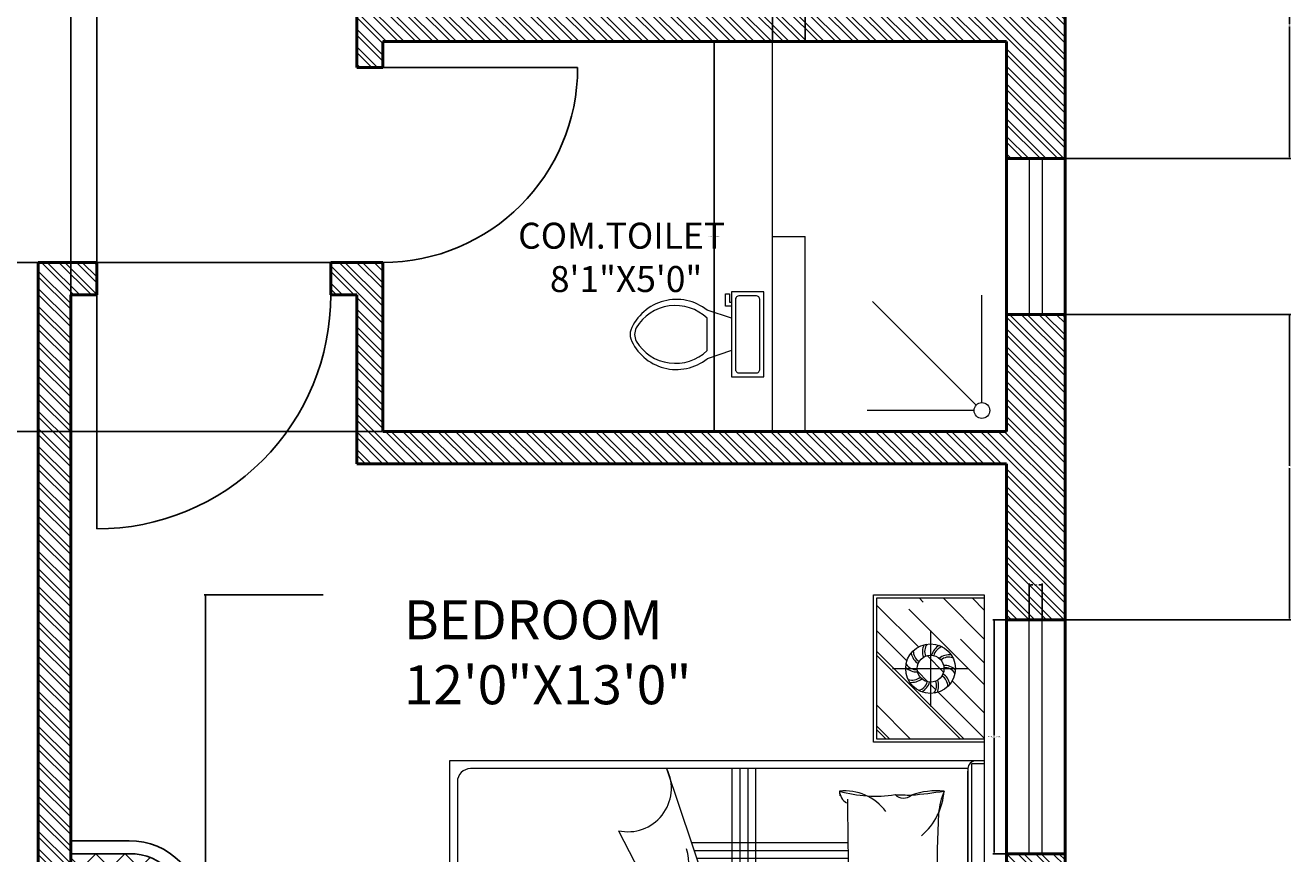
# Model space of a CAD drawing. Units: inches. Extents: x 10696 to 11614, y 5787 to 6498.
# Tile 3 of 9: x 10898 to 11093, y 5992 to 6120. Entities that reach past the tile are written whole.
import ezdxf

# ---------------------------------------------------------------- set-up
doc = ezdxf.new("R2010")
doc.units = ezdxf.units.IN
for name, color, linetype, lineweight in [('A-ANNO-DIMS', 2, 'Continuous', 18), ('A-AREA-IDEN', 7, 'Continuous', 25), ('A-DOOR', 3, 'Continuous', 25), ('A-FLOR-CASE', 32, 'Continuous', 25), ('A-FLOR-CASE-PATT', 252, 'Continuous', 13), ('A-FLOR-FIXT', 9, 'Continuous', 20), ('A-FURN', 8, 'Continuous', 18), ('A-GLAZ', 4, 'Continuous', 20), ('A-WALL', 7, 'Continuous', 50), ('A-WALL-PATT', 252, 'Continuous', 13)]:
    doc.layers.add(name, color=color, linetype=linetype, lineweight=lineweight)
doc.styles.get("Standard").update_dxf_attribs({"font": 'arial.ttf'})
doc.dimstyles.get("Standard").update_dxf_attribs({"dimtxt": 0.18, "dimasz": 0.18, "dimexe": 0.18, "dimexo": 0.0625, "dimgap": 0.09, "dimtad": 0, "dimtih": 1, "dimtoh": 1, "dimdec": 4, "dimzin": 0, "dimdsep": 46, "dimtxsty": 'Standard', "dimcen": 0.09, "dimadec": 0, "dimazin": 0, "dimtfac": 1, "dimtdec": 4, "dimtofl": 0, "dimtmove": 0, "dimatfit": 3, "dimfxl": 1, "dimtolj": 1, "dimtzin": 0, "dimarcsym": 0})

# ---------------------------------------------------------------- blocks, each defined once
blk = doc.blocks.new('A$C64B41DC1')
for p, q in [((0, 2.5079), (2.9903, 2.5079)), ((0, 2.0879), (0, 2.5079)), ((0.012, 2.4618), (0.0581, 2.5079)), ((0.012, 2.3515), (0.1684, 2.5079)), ((0.012, 2.0999), (0.012, 2.5079)), ((0.0543, 2.2213), (0.3409, 2.5079)), ((0.1689, 2.4179), (0.2589, 2.5079)), ((0.3265, 2.386), (0.4484, 2.5079)), ((0.3699, 2.3332), (0.5445, 2.5079)), ((0.548, 2.5079), (0.548, 2.0999)), ((0.56, 2.5079), (0.56, 2.0879)), ((0.6301, 2.5079), (0.6301, 0.4779)), ((0.6401, 2.461), (0.6401, 2.5079)), ((0.6401, 2.5079), (2.344, 2.5079)), ((2.344, 2.5079), (2.3601, 2.5079)), ((2.344, 2.5079), (2.344, 2.461)), ((2.3601, 2.5079), (2.3601, 2.4761)), ((2.3601, 0.4779), (2.3601, 2.5079)), ((2.4303, 2.5079), (2.4303, 2.0879)), ((2.4423, 2.5079), (2.4423, 2.0999)), ((2.4423, 2.3333), (2.6169, 2.5079)), ((2.4423, 2.2145), (2.7357, 2.5079)), ((2.705, 2.398), (2.8149, 2.5079)), ((2.7691, 2.3772), (2.8998, 2.5079)), ((2.7819, 2.3646), (2.9252, 2.5079)), ((2.9783, 2.0999), (2.9783, 2.5079)), ((2.9903, 2.0879), (2.9903, 2.5079)), ((2.344, 2.461), (0.6401, 2.461)), ((2.4423, 2.404), (2.5354, 2.4971)), ((0.2157, 2.0999), (0.548, 2.4322)), ((0.2299, 2.0999), (0.548, 2.418)), ((0.2804, 2.1597), (0.2804, 2.4481)), ((0.6601, 2.4461), (1.4951, 2.4461)), ((0.6601, 2.4461), (0.6601, 0.5579)), ((1.4951, 2.4461), (0.6697, 2.4461)), ((2.3301, 2.4461), (1.4951, 2.4461)), ((2.3301, 0.5579), (2.3301, 2.4461)), ((2.7099, 2.1597), (2.7099, 2.4481)), ((2.7914, 2.1846), (2.9783, 2.3715)), ((0.2311, 2.2906), (0.2937, 2.3532)), ((0.3405, 2.3039), (0.3605, 2.3238)), ((2.5849, 2.2779), (2.6158, 2.3088)), ((2.6158, 2.3088), (2.6313, 2.3243)), ((2.6674, 2.2756), (2.7382, 2.3464)), ((2.7249, 2.3076), (2.7512, 2.3339)), ((0.012, 2.261), (0.0275, 2.2765)), ((0.0404, 2.0999), (0.1982, 2.2578)), ((0.1362, 2.3039), (0.4246, 2.3039)), ((0.2905, 2.2539), (0.3304, 2.2938)), ((2.8541, 2.3039), (2.5657, 2.3039)), ((2.7746, 2.0999), (2.9783, 2.3036)), ((2.9144, 2.2312), (2.9783, 2.2951)), ((0.1365, 2.0999), (0.251, 2.2144)), ((0.4194, 2.0999), (0.548, 2.2285)), ((2.4423, 2.1353), (2.5382, 2.2312)), ((2.4918, 2.0999), (2.6366, 2.2447)), ((2.7831, 2.0999), (2.8678, 2.1846)), ((2.8962, 2.0999), (2.9783, 2.182)), ((0.4986, 2.0999), (0.548, 2.1493)), ((0.5127, 2.0999), (0.548, 2.1352)), ((0.56, 2.0879), (0, 2.0879)), ((0.548, 2.0999), (0.012, 2.0999)), ((2.4303, 2.0879), (2.9903, 2.0879)), ((2.4423, 2.0999), (2.9783, 2.0999)), ((2.5172, 2.0999), (2.5269, 2.1096)), ((0.9415, 1.9902), (0.9415, 1.3975)), ((0.9715, 1.9906), (0.9715, 1.4076)), ((1.0015, 1.991), (1.0015, 1.4177)), ((1.0315, 1.9916), (1.0315, 1.4279)), ((2.3349, 1.8678), (0.6613, 1.3029)), ((0.8956, 1.1191), (2.3349, 1.8678)), ((1.6636, 1.6412), (0.6601, 1.6412)), ((1.5748, 1.6112), (0.6601, 1.6112)), ((2.3665, 1.295), (2.3665, 1.3839)), ((2.377, 1.295), (2.3822, 1.3891)), ((2.4032, 1.295), (2.4032, 1.3839)), ((2.4346, 1.295), (2.4346, 1.3839)), ((2.4451, 1.295), (2.4503, 1.3891)), ((2.4774, 1.2957), (2.4774, 1.3837)), ((2.5, 1.295), (2.5, 1.3839)), ((2.5105, 1.295), (2.5157, 1.3891)), ((2.5367, 1.295), (2.5367, 1.3839)), ((2.5471, 1.295), (2.5524, 1.3891)), ((2.5681, 1.295), (2.5681, 1.3839)), ((2.5918, 1.295), (2.5918, 1.3839)), ((2.6346, 1.2957), (2.6346, 1.3837)), ((2.6362, 1.2957), (2.6467, 1.3839)), ((2.6729, 1.295), (2.6624, 1.3839)), ((2.6938, 1.295), (2.6938, 1.3839)), ((2.7043, 1.295), (2.7095, 1.3891)), ((2.7127, 1.2957), (2.7232, 1.3839)), ((2.7253, 1.295), (2.7253, 1.3839)), ((2.7494, 1.295), (2.7389, 1.3839)), ((2.7718, 1.295), (2.7718, 1.3839)), ((2.7959, 1.295), (2.7854, 1.3839)), ((2.8146, 1.2957), (2.8146, 1.3837)), ((2.8146, 1.2957), (2.8146, 1.3837)), ((2.8282, 1.295), (2.8282, 1.3839)), ((2.8282, 1.295), (2.8282, 1.3839)), ((2.8523, 1.295), (2.8418, 1.3839)), ((2.8523, 1.295), (2.8418, 1.3839)), ((2.8653, 1.2966), (2.8688, 1.3861)), ((2.8711, 1.2957), (2.8711, 1.3837)), ((2.8711, 1.2957), (2.8875, 1.3822)), ((2.8765, 1.2958), (2.9132, 1.3758)), ((2.8893, 1.3011), (2.9394, 1.3636)), ((2.8713, 1.2927), (2.954, 1.3315)), ((2.8717, 1.2884), (2.9588, 1.3058)), ((2.3601, 1.2873), (2.8639, 1.2873)), ((2.8639, 1.2873), (2.8639, 0.1018)), ((2.8716, 1.2565), (2.9605, 1.2669)), ((2.8723, 1.2489), (2.9603, 1.2489)), ((2.8744, 1.2817), (2.9603, 1.2869)), ((2.3601, 1.2233), (2.7999, 1.2233)), ((2.7999, 1.2233), (2.7999, 0.1658)), ((2.8716, 1.2212), (2.9605, 1.2212)), ((2.8716, 1.1947), (2.9605, 1.2052)), ((2.3601, 1.1913), (2.7679, 1.1912)), ((2.7679, 1.1912), (2.7679, 0.1978)), ((2.8716, 1.181), (2.9605, 1.1705)), ((2.8716, 1.1595), (2.9605, 1.1595)), ((2.8723, 1.1872), (2.9603, 1.1872)), ((2.8716, 1.133), (2.9605, 1.1435)), ((2.8716, 1.1193), (2.9605, 1.1088)), ((2.8723, 1.1255), (2.9603, 1.1255)), ((2.8716, 1.1035), (2.9605, 1.093)), ((2.8716, 1.0965), (2.9605, 1.0965)), ((2.8716, 1.086), (2.9657, 1.0913)), ((2.8716, 1.0756), (2.9605, 1.0756)), ((2.8716, 1.0491), (2.9605, 1.0596)), ((2.8723, 1.0858), (2.9605, 1.0753)), ((2.8716, 1.0354), (2.9605, 1.0249)), ((2.8723, 1.0416), (2.9603, 1.0416)), ((2.8723, 0.9987), (2.9605, 1.0092)), ((2.8723, 0.985), (2.9605, 0.9745)), ((2.8723, 0.9735), (2.9603, 0.9735)), ((2.8716, 0.9346), (2.9605, 0.9241)), ((2.8723, 0.9408), (2.9603, 0.9408)), ((2.8723, 0.8979), (2.9605, 0.9084)), ((2.8723, 0.8726), (2.9603, 0.8726)), ((2.8723, 0.8505), (2.9603, 0.8505)), ((2.8716, 0.7885), (2.9605, 0.799)), ((2.8716, 0.7818), (2.9657, 0.787)), ((2.8716, 0.7503), (2.9657, 0.7556)), ((2.8716, 0.7204), (2.9605, 0.7309)), ((2.8723, 0.7571), (2.9605, 0.7466)), ((2.8716, 0.6995), (2.9605, 0.6995)), ((2.8716, 0.689), (2.9657, 0.6838)), ((2.8716, 0.6576), (2.9657, 0.6523)), ((2.8716, 0.6471), (2.9605, 0.6471)), ((2.8716, 0.5903), (2.9605, 0.6007)), ((2.882, 0.5582), (2.9657, 0.5536)), ((0.7101, 0.5079), (2.2801, 0.5079)), ((2.8716, 0.4877), (2.9603, 0.4877)), ((2.8909, 0.5263), (2.9657, 0.5222)), ((2.8928, 0.5169), (2.9605, 0.5169)), ((0.6301, 0.4779), (2.3601, 0.4779)), ((1.2465, 0.4625), (1.1576, 0.452)), ((1.2465, 0.4365), (1.1577, 0.4365)), ((1.2542, 0.1018), (1.2542, 0.4779)), ((1.3182, 0.1658), (1.3182, 0.4779)), ((1.3502, 0.1978), (1.3502, 0.4779)), ((2.8716, 0.4625), (2.9605, 0.452)), ((2.8716, 0.4365), (2.9603, 0.4365)), ((1.2465, 0.3746), (1.1576, 0.3851)), ((2.8716, 0.3746), (2.9605, 0.3851)), ((1.2465, 0.3684), (1.1577, 0.3684)), ((2.8716, 0.3684), (2.9603, 0.3684)), ((1.2355, 0.3092), (1.1576, 0.3)), ((1.2285, 0.3357), (1.1577, 0.3357)), ((2.8826, 0.3092), (2.9605, 0.3)), ((2.8896, 0.3357), (2.9603, 0.3357)), ((1.2457, 0.2423), (1.1576, 0.2319)), ((1.2457, 0.2676), (1.1577, 0.2676)), ((2.8723, 0.2676), (2.9603, 0.2676)), ((2.8723, 0.2423), (2.9605, 0.2319)), ((1.2465, 0.2057), (1.1576, 0.2161)), ((2.7679, 0.1978), (1.3502, 0.1978)), ((2.8716, 0.2057), (2.9605, 0.2161)), ((1.2465, 0.1742), (1.1524, 0.169)), ((1.2465, 0.1847), (1.1576, 0.1847)), ((2.7999, 0.1658), (1.3182, 0.1658)), ((2.8716, 0.1847), (2.9605, 0.1847)), ((2.8716, 0.1742), (2.9657, 0.169)), ((1.2465, 0.1428), (1.1524, 0.1376)), ((1.2465, 0.1334), (1.1524, 0.1281)), ((1.2465, 0.1323), (1.1576, 0.1323)), ((1.2465, 0.1323), (1.1576, 0.1323)), ((1.2465, 0.1), (1.1576, 0.1105)), ((1.2465, 0.1229), (1.1588, 0.1168)), ((1.2464, 0.1007), (1.1592, 0.0833)), ((1.2468, 0.0964), (1.1641, 0.0576)), ((2.8639, 0.1018), (1.2542, 0.1018)), ((2.8713, 0.0964), (2.954, 0.0576)), ((2.8716, 0.1428), (2.9657, 0.1376)), ((2.8716, 0.1334), (2.9657, 0.1281)), ((2.8716, 0.1323), (2.9605, 0.1323)), ((2.8716, 0.1229), (2.9593, 0.1168)), ((2.8717, 0.1007), (2.9588, 0.0833)), ((2.8744, 0.1074), (2.9603, 0.1022)), ((1.2288, 0.088), (1.1787, 0.0255)), ((1.2415, 0.0933), (1.2049, 0.0133)), ((1.247, 0.0934), (1.2306, 0.0069)), ((1.2527, 0.0925), (1.2493, 0.003)), ((1.2658, 0.0941), (1.2762, 0.0052)), ((1.2899, 0.0941), (1.2899, 0.0052)), ((1.2999, 0.0941), (1.3051, 0)), ((1.3313, 0.0941), (1.3365, 0)), ((1.3523, 0.0941), (1.3575, 0)), ((1.3804, 0.0941), (1.3699, 0.0052)), ((1.4119, 0.0934), (1.4223, 0.0052)), ((1.4485, 0.0941), (1.438, 0.0052)), ((1.48, 0.0941), (1.4852, 0)), ((1.5114, 0.0941), (1.5166, 0)), ((1.5323, 0.0941), (1.5376, 0)), ((1.5638, 0.0941), (1.5638, 0.0105)), ((1.6021, 0.0941), (1.6021, 0.0052)), ((1.6336, 0.0941), (1.6336, 0.0052)), ((1.6702, 0.0941), (1.6702, 0.0052)), ((1.7017, 0.0941), (1.7017, 0.0052)), ((1.7122, 0.0941), (1.7174, 0)), ((1.7445, 0.0934), (1.7445, 0.0054)), ((1.7698, 0.0934), (1.7803, 0.0052)), ((1.8065, 0.0941), (1.796, 0.0052)), ((1.8274, 0.0941), (1.8274, 0.0052)), ((1.8379, 0.0941), (1.8431, 0)), ((1.8746, 0.0941), (1.8798, 0)), ((1.8955, 0.0941), (1.8955, 0.0052)), ((1.906, 0.0941), (1.9113, 0)), ((1.9384, 0.0934), (1.9384, 0.0054)), ((1.9609, 0.0941), (1.9609, 0.0052)), ((1.9636, 0.0934), (1.9741, 0.0052)), ((1.9714, 0.0941), (1.9766, 0)), ((1.9976, 0.0941), (1.9976, 0.0052)), ((2.0081, 0.0941), (2.0133, 0)), ((2.029, 0.0941), (2.029, 0.0052)), ((2.0395, 0.0941), (2.0447, 0)), ((2.0797, 0.0941), (2.0797, 0.0052)), ((2.0902, 0.0941), (2.0954, 0)), ((2.1216, 0.0941), (2.1269, 0)), ((2.1412, 0.0941), (2.1412, 0.0052)), ((2.1517, 0.0941), (2.1569, 0)), ((2.1831, 0.0941), (2.1884, 0)), ((2.2093, 0.0941), (2.2093, 0.0052)), ((2.2198, 0.0941), (2.225, 0)), ((2.2512, 0.0941), (2.2565, 0)), ((2.2603, 0.0934), (2.2707, 0.0052)), ((2.2969, 0.0941), (2.2864, 0.0052)), ((2.3089, 0.0934), (2.3193, 0.0052)), ((2.3455, 0.0941), (2.3351, 0.0052)), ((2.3665, 0.0941), (2.3665, 0.0052)), ((2.377, 0.0941), (2.3822, 0)), ((2.4032, 0.0941), (2.4032, 0.0052)), ((2.4346, 0.0941), (2.4346, 0.0052)), ((2.4451, 0.0941), (2.4503, 0)), ((2.4774, 0.0934), (2.4774, 0.0054)), ((2.5, 0.0941), (2.5, 0.0052)), ((2.5105, 0.0941), (2.5157, 0)), ((2.5367, 0.0941), (2.5367, 0.0052)), ((2.5471, 0.0941), (2.5524, 0)), ((2.5681, 0.0941), (2.5681, 0.0052)), ((2.5918, 0.0941), (2.5918, 0.0052)), ((2.6346, 0.0934), (2.6346, 0.0054)), ((2.6362, 0.0934), (2.6467, 0.0052)), ((2.6729, 0.0941), (2.6624, 0.0052)), ((2.6938, 0.0941), (2.6938, 0.0052)), ((2.7043, 0.0941), (2.7095, 0)), ((2.7127, 0.0934), (2.7232, 0.0052)), ((2.7253, 0.0941), (2.7253, 0.0052)), ((2.7494, 0.0941), (2.7389, 0.0052)), ((2.7718, 0.0941), (2.7718, 0.0052)), ((2.7959, 0.0941), (2.7854, 0.0052)), ((2.8146, 0.0934), (2.8146, 0.0054)), ((2.8282, 0.0941), (2.8282, 0.0052)), ((2.8523, 0.0941), (2.8418, 0.0052)), ((2.8653, 0.0925), (2.8688, 0.003)), ((2.8711, 0.0934), (2.8875, 0.0069)), ((2.8765, 0.0933), (2.9132, 0.0133)), ((2.8893, 0.088), (2.9394, 0.0255))]:
    blk.add_line(p, q)
at = {"ltscale": 10}
for p, q in [((1.4859, 1.5812), (0.6601, 1.5812)), ((1.397, 1.5512), (0.6601, 1.5512))]:
    blk.add_line(p, q, dxfattribs=at)
for centre, radius in [((0.2804, 2.3039), 0.0942), ((0.2804, 2.3039), 0.051), ((2.7099, 2.3039), 0.0942), ((2.7099, 2.3039), 0.051)]:
    blk.add_circle(centre, radius)
for centre, radius, start, end in [((0.6601, 2.4761), 0.03, 180, 270), ((2.3301, 2.4761), 0.03, 270, 0), ((0.2887, 2.3745), 0.0605, 172.17, 218.4897), ((0.2828, 2.3731), 0.0462, 160.3002, 220.538), ((0.3286, 2.3561), 0.0605, 136.17, 182.4897), ((0.3231, 2.3585), 0.0462, 124.3002, 184.538), ((0.3501, 2.3178), 0.0605, 100.17, 146.4897), ((0.347, 2.323), 0.0462, 88.3002, 148.538), ((1.0526, 2.3302), 0.3085, 175.3048, 198.6942), ((-0.8702, 2.0941), 1.6364, 4.8098, 9.1892), ((0.8579, 2.6278), 0.2948, 247.5179, 264.267), ((0.728, 2.111), 0.245, 40.4189, 85.9871), ((1.6986, 2.3355), 0.1943, 174.11, 233.4289), ((1.1481, 2.2311), 0.3783, 353.4947, 19.1867), ((1.6871, 3.192), 0.8561, 257.7438, 273.6284), ((1.4882, 2.111), 0.245, 40.4189, 85.9871), ((1.8674, 1.9709), 0.3878, 68.2026, 108.9817), ((2.6433, 2.323), 0.0462, 31.462, 91.6998), ((2.6402, 2.3178), 0.0605, 33.5103, 79.83), ((2.6672, 2.3585), 0.0462, 355.462, 55.6998), ((2.6617, 2.3561), 0.0605, 357.5103, 43.83), ((2.7075, 2.3731), 0.0462, 319.462, 19.6998), ((2.7016, 2.3745), 0.0605, 321.5103, 7.83), ((0.2457, 2.3659), 0.0605, 208.17, 254.4897), ((0.2417, 2.3614), 0.0462, 196.3002, 256.538), ((0.3449, 2.2742), 0.0605, 64.17, 110.4897), ((0.3455, 2.2802), 0.0462, 52.3002, 112.538), ((1.0164, 5.7096), 3.3803, 266.8134, 276.1602), ((1.3963, 2.1044), 0.245, 94.0129, 139.5811), ((1.1858, 2.3288), 0.1943, 306.5711, 5.89), ((1.5348, 2.2652), 0.1767, 151.7736, 201.6983), ((2.1269, 2.1044), 0.245, 94.0129, 139.5811), ((2.0342, 2.4856), 0.1563, 261.5958, 298.9092), ((1.9165, 2.3288), 0.1943, 333.7371, 5.89), ((2.6058, 2.2028), 0.517, 163.6046, 172.3273), ((2.6448, 2.2802), 0.0462, 67.462, 127.6998), ((2.6454, 2.2742), 0.0605, 69.5103, 115.83), ((2.7486, 2.3614), 0.0462, 283.462, 343.6998), ((2.7446, 2.3659), 0.0605, 285.5103, 331.83), ((0.2153, 2.3276), 0.0462, 232.3002, 292.538), ((0.2158, 2.3336), 0.0605, 244.17, 290.4897), ((0.2138, 2.2848), 0.0462, 268.3002, 328.538), ((0.2779, 2.2347), 0.0462, 340.3002, 40.538), ((0.272, 2.2333), 0.0605, 352.17, 38.4897), ((0.3191, 2.2464), 0.0462, 16.3002, 76.538), ((0.3151, 2.2419), 0.0605, 28.17, 74.4897), ((2.6752, 2.2419), 0.0605, 105.5103, 151.83), ((2.6712, 2.2464), 0.0462, 103.462, 163.6998), ((2.7182, 2.2333), 0.0605, 141.5103, 187.83), ((2.7123, 2.2347), 0.0462, 139.462, 199.6998), ((2.7765, 2.2848), 0.0462, 211.462, 271.6998), ((2.7744, 2.3336), 0.0605, 249.5103, 295.83), ((2.775, 2.3276), 0.0462, 247.462, 307.6998), ((0.2107, 2.29), 0.0605, 280.17, 326.4897), ((0.2377, 2.2493), 0.0462, 304.3002, 4.538), ((0.2322, 2.2517), 0.0605, 316.17, 2.4897), ((0.7274, 2.2013), 0.0446, 314.4736, 42.1713), ((-1.6008, 2.277), 2.3618, 357.3905, 358.8876), ((1.9165, 2.3288), 0.1943, 320.9404, 333.7371), ((2.1347, 2.2313), 0.0459, 165.3506, 223.2684), ((2.7581, 2.2517), 0.0605, 177.5103, 223.83), ((2.7526, 2.2493), 0.0462, 175.462, 235.6998), ((2.7796, 2.29), 0.0605, 213.5103, 259.83), ((0.2688, 2.0945), 0.4956, 344.0243, 8.7071), ((1.204, 2.1778), 0.1681, 337.017, 7.5368), ((1.5671, 2.1546), 0.0547, 142.0833, 220.902), ((1.9346, 2.1778), 0.1681, 337.017, 7.5368), ((0.9385, 1.978), 0.1943, 126.5711, 185.89), ((1.1858, 1.9714), 0.1943, 4.3181, 53.4289), ((1.7059, 1.9714), 0.204, 127.1197, 175.09), ((1.1965, 2.0983), 0.3299, 343.7954, 3.5554), ((1.9394, 1.991), 0.1651, 351.2621, 55.7572), ((1.5415, 2.0969), 0.1834, 175.2233, 196.23), ((2.4617, 2.0719), 0.3745, 173.8296, 196.4356), ((1.2687, 1.9248), 0.1223, 33.628, 86.4744), ((1.7676, 1.0629), 0.9631, 69.6507, 105.9631), ((2.2748, 2.5795), 0.6373, 238.3499, 254.3137), ((0.7417, 2.0149), 0.057, 273.4709, 328.5412), ((0.7246, 18.8439), 16.8552, 270.17399, 272.05214), ((1.3401, 1.9404), 0.0603, 49.0991, 101.3702), ((2.0911, 2.0123), 0.0478, 179.7727, 283.8018), ((0.728, 2.2025), 0.245, 274.0129, 278.3417), ((1.0747, 1.2871), 0.1871, 14.1863, 69.1212), ((1.0274, 1.1334), 0.2527, 40.629, 104.3712), ((0.7347, 1.1553), 0.1649, 347.3109, 116.4454), ((0.7101, 0.5579), 0.05, 180, 270), ((2.2801, 0.5579), 0.05, 270, 0)]:
    blk.add_arc(centre, radius, start, end)
for centre, major_axis, ratio, start_param, end_param in [((1.9938, 1.6262), (0, -0.7531), 0.68, 0.797284, 0.954936), ((2.0643, 1.466), (0, -0.5322), 0.68, 7.239912, 7.311536), ((1.9052, 1.7397), (0, -0.9842), 0.68, 0.74745, 0.979724), ((2.7455, 1.3081), (0, 0.3614), 0.68, 1.900046, 2.742661), ((2.7868, 1.3081), (0, 0.3614), 0.68, 1.900046, 2.614747), ((2.8372, 1.3081), (0, 0.3614), 0.68, 1.900046, 2.479658), ((2.8607, 1.3211), (0, 0.3614), 0.68, 1.938265, 2.479658), ((2.8057, 1.2079), (0, -0.1524), 0.68, 4.821745, 5.895886), ((2.4665, 0.8216), (0, -0.2664), 0.68, 2.006169, 3.565187), ((2.4513, 0.5069), (0, 0.502), 0.68, 5.095327, 6.553458), ((2.7862, 0.8069), (0, -0.2615), 0.68, 3.244645, 4.205018), ((2.396, 0.6032), (0, 0.3641), 0.68, -1.3172, 0.145284), ((2.7784, 0.8289), (0, -0.1802), 0.68, 3.227058, 4.318474), ((2.3507, 0.5642), (0.0073, 0.3819), 0.56205, -1.21172, -0.009991), ((2.7821, 0.7971), (0, -0.1589), 0.68, 3.272942, 4.229533), ((2.2964, 0.5771), (0, -0.3263), 0.68, 1.938944, 2.850232), ((2.0403, 1.6015), (0, -0.8763), 0.68, 6.849801, 6.887077), ((2.4005, 0.7132), (0, -0.1214), 0.68, 2.284368, 3.652258), ((2.3834, 0.7081), (0, 0.1147), 0.68, 4.593909, 6.585576), ((2.3961, 0.7628), (0, -0.0317), 0.68, 1.462497, 5.046281), ((2.3774, 0.7653), (0, -0.0593), 0.68, 5.841311, 7.755362), ((1.9938, 1.1295), (-0.0678, 0.7439), 0.610498, 3.917146, 4.063997), ((2.0643, 0.9693), (0, -0.5322), 0.68, 7.239912, 7.336618), ((1.9052, 1.243), (0, -0.9842), 0.68, 0.74745, 0.979724), ((2.7455, 0.8114), (-0.0599, 0.3735), 0.695517, 1.775813, 2.548612), ((2.7868, 0.8114), (0, 0.3614), 0.68, 1.900046, 2.614747), ((2.8607, 0.8243), (0, 0.3614), 0.68, 1.938265, 2.479658), ((2.4665, 0.3249), (0, -0.2664), 0.68, 2.006169, 3.565187), ((2.4513, 0.0102), (0, 0.502), 0.68, 5.095327, 6.553458), ((2.7862, 0.3102), (0, -0.2615), 0.68, 3.244645, 4.205018), ((1.5283, 0.0674), (0, -0.3703), 0.68, 1.930561, 3.464283), ((1.5736, 0.1065), (0, 0.3641), 0.68, -1.3172, 0.476403), ((2.3507, 0.0674), (0, -0.3703), 0.68, 1.930561, 3.464283), ((2.396, 0.1065), (0, 0.3641), 0.68, -1.3172, 0.476403), ((2.7784, 0.3322), (0, -0.1802), 0.68, 3.227058, 4.318474), ((1.242, 0.9693), (0, -0.5322), 0.68, 6.586764, 6.677612), ((1.1714, 1.1295), (-0.1157, 0.7241), 0.59432, 3.291697, 3.50733), ((1.0828, 1.243), (0, -0.9842), 0.68, 0.565948, 0.680366), ((1.6289, 0.0102), (0, 0.502), 0.68, 6.655152, 6.661293), ((1.6289, 0.0102), (0, 0.502), 0.68, 5.095327, 5.911219), ((1.6442, 0.3249), (0, -0.2664), 0.68, 2.006169, 2.182797), ((1.9638, 0.3102), (0, -0.2615), 0.68, 4.015924, 4.205018), ((1.956, 0.3322), (0, -0.1802), 0.68, 3.770744, 4.318474), ((1.9597, 0.3004), (0, -0.1589), 0.68, 3.14258, 4.229533), ((2.0606, 0.5616), (0, -0.1803), 0.68, 5.194792, 5.929328), ((2.0606, 0.5616), (0, -0.1803), 0.68, 5.194792, 6.723255), ((2.1315, 0.6603), (0, -0.3155), 0.68, 5.328638, 6.949396), ((2.0549, 0.5656), (0, -0.1303), 0.68, 5.450951, 6.054641), ((2.0643, 0.9693), (0, -0.5322), 0.68, 6.20013, 6.677612), ((1.9938, 1.1295), (-0.0678, 0.7439), 0.610498, 3.199135, 3.592282), ((1.9052, 1.243), (0, -0.9842), 0.68, 0.565948, 0.680366), ((2.4513, 0.0102), (0, 0.502), 0.68, 6.655152, 6.661293), ((2.7821, 0.3004), (0, -0.1589), 0.68, 3.272942, 4.229533), ((1.1933, 0.9181), (0, -0.624), 0.68, 0.378672, 0.625379), ((1.3091, 0.6603), (0, -0.3155), 0.68, 6.475719, 6.949396), ((1.1911, 1.1066), (0, 0.8458), 0.68, 3.421828, 3.728616), ((1.474, 0.0804), (0, -0.3263), 0.68, 1.938944, 3.339184), ((2.0157, 0.9181), (0, -0.624), 0.68, -0.280078, 0.625379), ((2.0135, 1.1066), (0, 0.8458), 0.68, 2.978727, 3.728616), ((2.2964, 0.0804), (0, -0.3263), 0.68, 1.938944, 3.339184), ((1.2179, 1.1047), (0, -0.8763), 0.68, 6.507006, 6.887077), ((1.5781, 0.2165), (0, -0.1214), 0.68, 2.284368, 3.726131), ((2.0403, 1.1047), (0, -0.8763), 0.68, 6.099302, 6.887077), ((2.4005, 0.2165), (0, -0.1214), 0.68, 2.284368, 3.726131), ((1.555, 0.2685), (0, -0.0593), 0.68, 3.732151, 7.755362), ((1.561, 0.2114), (0, 0.1147), 0.68, 4.593909, 6.647252), ((1.5737, 0.2661), (0, -0.0317), 0.68, 1.462497, 5.046281), ((2.3774, 0.2685), (0, -0.0593), 0.68, 3.732151, 7.755362), ((2.3834, 0.2114), (0, 0.1147), 0.68, 4.593909, 6.647252), ((2.3961, 0.2661), (0, -0.0317), 0.68, 1.462497, 5.046281)]:
    blk.add_ellipse(centre, major_axis=major_axis, ratio=ratio, start_param=start_param, end_param=end_param)
blk = doc.blocks.new('*U10')
for p, q in [((9.5, -6), (9.5, -2)), ((-10, -8.5), (-8, -8.5)), ((-10, -9.5), (-10, -8.5)), ((-8, -8.5), (-8, -8)), ((-7, -8), (-7, -9.5)), ((-4, -8), (-6, -14)), ((4, -8), (6, -14)), ((-7, -9.5), (-10, -9.5)), ((4, -14), (-4, -14))]:
    blk.add_line(p, q)
blk.add_lwpolyline([(10.5, -8), (10.5, 0), (-10.5, 0), (-10.5, -8)], close=True)
for points in [[(-9.5, -2), (-9.5, -6)], [(8.5, -1), (-8.5, -1)], [(-8.5, -7), (8.5, -7)]]:
    blk.add_lwpolyline(points)
for centre, radius, start, end in [((-8.62, -1.88), 0.884, 81.8699, 188.1301), ((8.62, -1.88), 0.884, 351.8699, 98.1301), ((-8.62, -6.12), 0.884, 171.8699, 278.1301), ((8.62, -6.12), 0.884, 261.8699, 8.1301), ((3.52, -21.58), 12.17, 141.4691, 247.9714), ((4.2, -21.82), 11.33, 136.3677, 238.9468), ((-3.52, -21.58), 12.17, 292.0284, 38.5307), ((-4.2, -21.82), 11.33, 301.053, 43.6321), ((0, -27.88), 4, 245.7318, 294.2682), ((0, -29), 4, 254.8605, 285.1395)]:
    blk.add_arc(centre, radius, start, end)
blk = doc.blocks.new('DOOR-SINGLE-30')
blk.add_line((0, 30), (30, 30))
blk.add_arc((0, 30), 30, 270, 0)
blk = doc.blocks.new('DOOR-SINGLE-36-BEDROOM')
blk.add_line((0, 36), (0, 0))
blk.add_arc((0.1, 35.9), 35.9, 269.8411, 0.1589)
blk = doc.blocks.new('WIN-GLAZ-24')
for p, q in [((0, 24), (0, 0)), ((2, 24), (2, 0))]:
    blk.add_line(p, q)
blk = doc.blocks.new('WIN-GLAZ-36')
for p, q in [((0, 0), (0, 36)), ((2, 0), (2, 36))]:
    blk.add_line(p, q)
blk = doc.blocks.new('SHOWER-SCREEN')
for p, q in [((0, 0), (0, 60)), ((0, 30), (5, 30)), ((5, 0), (5, 30))]:
    blk.add_line(p, q)
blk = doc.blocks.new('SHOWER-DRAIN')
for p, q in [((16.81, 2.05), (0.86, 18)), ((17.68, 2.42), (17.68, 18.95)), ((16.47, 1.21), (0, 1.21))]:
    blk.add_line(p, q)
blk.add_circle((17.68, 1.21), 1.21)
blk = doc.blocks.new('*D34')
at = {"layer": 'A-ANNO-DIMS', "color": 0, "lineweight": -2, "transparency": 16777216}
for p, q in [((11052.35, 6028.07), (11046.83, 6028.07)), ((11047.01, 6027.89), (11047.01, 6010.25)), ((11047.01, 5992.25), (11047.01, 6009.89)), ((11052.35, 5992.07), (11046.83, 5992.07))]:
    blk.add_line(p, q, dxfattribs=at)
at = {"layer": 'A-ANNO-DIMS', "color": 0, "transparency": 16777216}
for points in [[(11046.98, 6027.89), (11047.04, 6027.89), (11047.01, 6028.07)], [(11046.98, 5992.25), (11047.04, 5992.25), (11047.01, 5992.07)]]:
    blk.add_solid(points, dxfattribs=at)
at = {"layer": 'Defpoints', "color": 0, "transparency": 16777216}
for p in [(11047.01, 6028.07), (11052.41, 6028.07), (11052.41, 5992.07)]:
    blk.add_point(p, dxfattribs=at)
at = {"layer": 'A-ANNO-DIMS', "color": 0, "transparency": 16777216, "insert": (11047.01, 6010.07), "char_height": 0.18, "attachment_point": 5}
blk.add_mtext('\\A1;WINDOW 36 TYP.', dxfattribs=at)
blk = doc.blocks.new('*D35')
at = {"layer": 'A-ANNO-DIMS', "color": 0, "lineweight": -2, "transparency": 16777216}
for p, q in [((11052.41, 6028.13), (11052.41, 6033.65)), ((11052.59, 6033.47), (11052.95, 6033.47)), ((11054.23, 6033.47), (11053.87, 6033.47)), ((11054.41, 6028.13), (11054.41, 6033.65))]:
    blk.add_line(p, q, dxfattribs=at)
at = {"layer": 'A-ANNO-DIMS', "color": 0, "transparency": 16777216}
for points in [[(11052.59, 6033.5), (11052.59, 6033.44), (11052.41, 6033.47)], [(11054.23, 6033.5), (11054.23, 6033.44), (11054.41, 6033.47)]]:
    blk.add_solid(points, dxfattribs=at)
at = {"layer": 'Defpoints', "color": 0, "transparency": 16777216}
for p in [(11054.41, 6033.47), (11052.41, 6028.07), (11054.41, 6028.07)]:
    blk.add_point(p, dxfattribs=at)
at = {"layer": 'A-ANNO-DIMS', "color": 0, "transparency": 16777216, "insert": (11053.41, 6033.47), "char_height": 0.18, "attachment_point": 5}
blk.add_mtext('\\A1;2 TYP.', dxfattribs=at)
blk = doc.blocks.new('*D42')
at = {"layer": 'A-ANNO-DIMS', "color": 0, "lineweight": -2, "transparency": 16777216}
for p, q in [((10943.75, 6031.92), (10925.45, 6031.92)), ((10925.63, 6031.74), (10925.63, 5971.49)), ((10925.63, 5910.87), (10925.63, 5971.12)), ((10943.75, 5910.69), (10925.45, 5910.69))]:
    blk.add_line(p, q, dxfattribs=at)
at = {"layer": 'A-ANNO-DIMS', "color": 0, "transparency": 16777216}
for points in [[(10925.6, 6031.74), (10925.66, 6031.74), (10925.63, 6031.92)], [(10925.6, 5910.87), (10925.66, 5910.87), (10925.63, 5910.69)]]:
    blk.add_solid(points, dxfattribs=at)
at = {"layer": 'Defpoints', "color": 0, "transparency": 16777216}
for p in [(10943.82, 6031.92), (10925.63, 5910.69), (10943.82, 5910.69)]:
    blk.add_point(p, dxfattribs=at)
at = {"layer": 'A-ANNO-DIMS', "color": 0, "transparency": 16777216, "insert": (10925.63, 5971.31), "char_height": 0.18, "attachment_point": 5}
blk.add_mtext('\\A1;BED GROUP 121 TYP.', dxfattribs=at)
blk = doc.blocks.new('*D60')
at = {"layer": 'A-ANNO-DIMS', "color": 0, "lineweight": -2, "transparency": 16777216}
for p, q in [((11012.85, 6117.07), (11003.73, 6117.07)), ((11003.91, 6116.89), (11003.91, 6087.25)), ((11003.91, 6057.25), (11003.91, 6086.89)), ((11012.85, 6057.07), (11003.73, 6057.07))]:
    blk.add_line(p, q, dxfattribs=at)
at = {"layer": 'A-ANNO-DIMS', "color": 0, "transparency": 16777216}
for points in [[(11003.88, 6116.89), (11003.94, 6116.89), (11003.91, 6117.07)], [(11003.88, 6057.25), (11003.94, 6057.25), (11003.91, 6057.07)]]:
    blk.add_solid(points, dxfattribs=at)
at = {"layer": 'Defpoints', "color": 0, "transparency": 16777216}
for p in [(11003.91, 6117.07), (11012.91, 6117.07), (11012.91, 6057.07)]:
    blk.add_point(p, dxfattribs=at)
at = {"layer": 'A-ANNO-DIMS', "color": 0, "transparency": 16777216, "insert": (11003.91, 6087.07), "char_height": 0.18, "attachment_point": 5}
blk.add_mtext('\\A1;SCREEN 60 TYP.', dxfattribs=at)
blk = doc.blocks.new('*D61')
at = {"layer": 'A-ANNO-DIMS', "color": 0, "lineweight": -2, "transparency": 16777216}
for p, q in [((11012.91, 6117.13), (11012.91, 6126.25)), ((11017.91, 6117.13), (11017.91, 6126.25)), ((11013.09, 6126.07), (11014.95, 6126.07)), ((11017.73, 6126.07), (11015.87, 6126.07))]:
    blk.add_line(p, q, dxfattribs=at)
at = {"layer": 'A-ANNO-DIMS', "color": 0, "transparency": 16777216}
for points in [[(11013.09, 6126.1), (11013.09, 6126.04), (11012.91, 6126.07)], [(11017.73, 6126.1), (11017.73, 6126.04), (11017.91, 6126.07)]]:
    blk.add_solid(points, dxfattribs=at)
at = {"layer": 'Defpoints', "color": 0, "transparency": 16777216}
for p in [(11017.91, 6126.07), (11012.91, 6117.07), (11017.91, 6117.07)]:
    blk.add_point(p, dxfattribs=at)
at = {"layer": 'A-ANNO-DIMS', "color": 0, "transparency": 16777216, "insert": (11015.41, 6126.07), "char_height": 0.18, "attachment_point": 5}
blk.add_mtext('\\A1;5 TYP.', dxfattribs=at)
blk = doc.blocks.new('*D88')
at = {"layer": 'A-ANNO-DIMS', "color": 0, "lineweight": -2, "transparency": 16777216}
for p, q in [((11057.975441, 6075.07026), (11092.642941, 6075.07026)), ((11092.462941, 6074.89026), (11092.462941, 6051.75026)), ((11092.462941, 6028.25026), (11092.462941, 6051.39026)), ((11057.975441, 6028.07026), (11092.642941, 6028.07026))]:
    blk.add_line(p, q, dxfattribs=at)
at = {"layer": 'A-ANNO-DIMS', "color": 0, "transparency": 16777216}
for points in [[(11092.432941, 6074.89026), (11092.492941, 6074.89026), (11092.462941, 6075.07026)], [(11092.432941, 6028.25026), (11092.492941, 6028.25026), (11092.462941, 6028.07026)]]:
    blk.add_solid(points, dxfattribs=at)
at = {"layer": 'Defpoints', "color": 0, "transparency": 16777216}
for p in [(11057.912941, 6075.07026), (11092.462941, 6075.07026), (11057.912941, 6028.07026)]:
    blk.add_point(p, dxfattribs=at)
at = {"layer": 'A-ANNO-DIMS', "color": 0, "transparency": 16777216, "insert": (11092.462941, 6051.57026), "char_height": 0.18, "attachment_point": 5}
blk.add_mtext('\\A1;47', dxfattribs=at)
blk = doc.blocks.new('*D89')
at = {"layer": 'A-ANNO-DIMS', "color": 0, "lineweight": -2, "transparency": 16777216}
for p, q in [((11057.98, 6140.07), (11092.64, 6140.07)), ((11092.46, 6139.89), (11092.46, 6119.75)), ((11092.46, 6099.25), (11092.46, 6119.39)), ((11057.98, 6099.07), (11092.64, 6099.07))]:
    blk.add_line(p, q, dxfattribs=at)
at = {"layer": 'A-ANNO-DIMS', "color": 0, "transparency": 16777216}
for points in [[(11092.43, 6139.89), (11092.49, 6139.89), (11092.46, 6140.07)], [(11092.43, 6099.25), (11092.49, 6099.25), (11092.46, 6099.07)]]:
    blk.add_solid(points, dxfattribs=at)
at = {"layer": 'Defpoints', "color": 0, "transparency": 16777216}
for p in [(11057.91, 6140.07), (11092.46, 6140.07), (11057.91, 6099.07)]:
    blk.add_point(p, dxfattribs=at)
at = {"layer": 'A-ANNO-DIMS', "color": 0, "transparency": 16777216, "insert": (11092.46, 6119.57), "char_height": 0.18, "attachment_point": 5}
blk.add_mtext('\\A1;41', dxfattribs=at)
blk = doc.blocks.new('*D98')
at = {"layer": 'A-ANNO-DIMS', "color": 0, "lineweight": -2, "transparency": 16777216}
for p, q in [((10952.85, 6083.07), (10696.18, 6083.07)), ((10696.36, 6082.89), (10696.36, 6070.25)), ((10696.36, 6057.25), (10696.36, 6069.89)), ((10952.85, 6057.07), (10696.18, 6057.07))]:
    blk.add_line(p, q, dxfattribs=at)
at = {"layer": 'A-ANNO-DIMS', "color": 0, "transparency": 16777216}
for points in [[(10696.33, 6082.89), (10696.39, 6082.89), (10696.36, 6083.07)], [(10696.33, 6057.25), (10696.39, 6057.25), (10696.36, 6057.07)]]:
    blk.add_solid(points, dxfattribs=at)
at = {"layer": 'Defpoints', "color": 0, "transparency": 16777216}
for p in [(10952.91, 6083.07), (10696.36, 6057.07), (10952.91, 6057.07)]:
    blk.add_point(p, dxfattribs=at)
at = {"layer": 'A-ANNO-DIMS', "color": 0, "transparency": 16777216, "insert": (10696.36, 6070.07), "char_height": 0.18, "attachment_point": 5}
blk.add_mtext('\\A1;26', dxfattribs=at)
blk = doc.blocks.new('*D100')
at = {"layer": 'A-ANNO-DIMS', "color": 0, "lineweight": -2, "transparency": 16777216}
for p, q in [((10904.91, 6078.13), (10904.91, 6497.62)), ((10905.09, 6497.44), (10906.76, 6497.44)), ((10908.73, 6497.44), (10907.07, 6497.44)), ((10908.91, 6078.13), (10908.91, 6497.62))]:
    blk.add_line(p, q, dxfattribs=at)
at = {"layer": 'A-ANNO-DIMS', "color": 0, "transparency": 16777216}
for points in [[(10905.09, 6497.47), (10905.09, 6497.41), (10904.91, 6497.44)], [(10908.73, 6497.47), (10908.73, 6497.41), (10908.91, 6497.44)]]:
    blk.add_solid(points, dxfattribs=at)
at = {"layer": 'Defpoints', "color": 0, "transparency": 16777216}
for p in [(10908.91, 6497.44), (10904.91, 6078.07), (10908.91, 6078.07)]:
    blk.add_point(p, dxfattribs=at)
at = {"layer": 'A-ANNO-DIMS', "color": 0, "transparency": 16777216, "insert": (10906.91, 6497.44), "char_height": 0.18, "attachment_point": 5}
blk.add_mtext('\\A1;4', dxfattribs=at)

msp = doc.modelspace()

# ---------------------------------------------------------------- hatches: boundary and pattern name
at = {"layer": 'A-FLOR-CASE-PATT'}
h = msp.add_hatch(dxfattribs=at)
h.set_pattern_fill('ANSI37', color=256)
h.paths.add_polyline_path([(10922.913, 5983.07, 0.4142136), (10913.913, 5992.07), (10904.913, 5992.07), (10904.913, 5896.07), (10922.913, 5896.07)])
h.paths.add_polyline_path([(10916.11, 5930.013), (10911.36, 5930.013), (10911.36, 5959.701), (10916.11, 5959.701)], flags=16)
at = {"layer": 'A-WALL-PATT'}
h = msp.add_hatch(dxfattribs=at)
h.set_pattern_fill('ANSI32', color=256, scale=0.2, angle=90)
h.paths.add_polyline_path([(10767.913, 5961.07), (10739.913, 5961.07), (10739.913, 6001.333), (10730.913, 6001.333), (10730.913, 5887.07), (10739.913, 5887.07), (10739.913, 5952.07), (10767.913, 5952.07)])
h.paths.add_polyline_path([(10739.913, 6127.055), (10730.913, 6127.055), (10730.913, 6073.333), (10739.913, 6073.333)])
h.paths.add_polyline_path([(10739.913, 6267.869, -0.035413), (10740.694, 6278.876), (10731.784, 6280.146, 0.035413), (10730.913, 6267.869), (10730.913, 6199.055), (10739.913, 6199.055)])
h.paths.add_polyline_path([(10794.29, 6342.205), (10791.564, 6350.783, 0.1142038), (10757.817, 6330.777), (10764.034, 6324.269, -0.1142038)])
h.paths.add_polyline_path([(10844.262, 6350.783), (10841.536, 6342.205, -0.065871), (10860.057, 6333.503), (10864.919, 6341.077, 0.065871)])
h.paths.add_polyline_path([(10908.913, 6311.07), (10895.913, 6311.07), (10895.913, 6306.404, 0.0519949), (10886.285, 6321.667), (10879.212, 6316.101, -0.1682272), (10895.913, 6267.869), (10895.913, 6223.07), (10904.913, 6223.07), (10904.913, 6302.07), (10908.913, 6302.07)])
h.paths.add_polyline_path([(11057.913, 6311.07), (10944.913, 6311.07), (10944.913, 6302.07), (11048.913, 6302.07), (11048.913, 6273.514), (11057.913, 6273.514)])
h.paths.add_polyline_path([(11057.913, 6225.514), (11048.913, 6225.514), (11048.913, 6187.07), (10988.913, 6187.07), (10988.913, 6182.07), (11048.913, 6182.07), (11048.913, 6164.07), (11057.913, 6164.07)])
h.paths.add_polyline_path([(10952.913, 6187.07), (10895.913, 6187.07), (10895.913, 6182.07), (10948.913, 6182.07), (10948.913, 6113.07), (10952.913, 6113.07), (10952.913, 6117.07), (11048.913, 6117.07), (11048.913, 6099.07), (11057.913, 6099.07), (11057.913, 6140.07), (11048.913, 6140.07), (11048.913, 6122.07), (10952.913, 6122.07)])
h.paths.add_polyline_path([(11057.913, 6075.07), (11048.913, 6075.07), (11048.913, 6057.07), (10952.913, 6057.07), (10952.913, 6083.07), (10944.913, 6083.07), (10944.913, 6078.07), (10948.913, 6078.07), (10948.913, 6052.07), (11048.913, 6052.07), (11048.913, 6028.07), (11057.913, 6028.07)])
h.paths.add_polyline_path([(11057.913, 5992.07), (11048.913, 5992.07), (11048.913, 5896.07), (11000.913, 5896.07), (11000.913, 5887.07), (11057.913, 5887.07)])
h.paths.add_polyline_path([(10952.913, 5896.07), (10904.913, 5896.07), (10904.913, 6078.07), (10908.913, 6078.07), (10908.913, 6083.07), (10899.913, 6083.07), (10899.913, 5961.07), (10891.913, 5961.07), (10891.913, 5952.07), (10895.913, 5952.07), (10895.913, 5887.07), (10952.913, 5887.07)])
h.paths.add_polyline_path([(10843.913, 5961.07), (10815.913, 5961.07), (10815.913, 5952.07), (10843.913, 5952.07)])

# ---------------------------------------------------------------- linework, layer by layer
at = {"layer": 'A-FLOR-CASE'}
for p, q in [((10904.913, 5994.07), (10913.913, 5994.07)), ((10904.913, 5992.07), (10913.913, 5992.07))]:
    msp.add_line(p, q, dxfattribs=at)
for radius in [11, 9]:
    msp.add_arc((10913.913, 5983.07), radius, 0, 90, dxfattribs=at)
at = {"layer": 'A-WALL'}
for p, q in [((11057.913, 5887.07), (11057.913, 6311.07)), ((10948.913, 6113.07), (10948.913, 6182.07)), ((10952.913, 6117.07), (11048.913, 6117.07)), ((10952.913, 6113.07), (10952.913, 6117.07)), ((11048.913, 6057.07), (11048.913, 6117.07)), ((10948.913, 6113.07), (10952.913, 6113.07)), ((11048.913, 6099.07), (11057.913, 6099.07)), ((10899.913, 5961.07), (10899.913, 6083.07)), ((10899.913, 6083.07), (10908.913, 6083.07)), ((10908.913, 6078.07), (10908.913, 6083.07)), ((10944.913, 6078.07), (10944.913, 6083.07)), ((10944.913, 6083.07), (10952.913, 6083.07)), ((10952.913, 6057.07), (10952.913, 6083.07)), ((10904.913, 5896.07), (10904.913, 6078.07)), ((10904.913, 6078.07), (10908.913, 6078.07)), ((10944.913, 6078.07), (10948.913, 6078.07)), ((10948.913, 6052.07), (10948.913, 6078.07)), ((11048.913, 6075.07), (11057.913, 6075.07)), ((10952.913, 6057.07), (11048.913, 6057.07)), ((10948.913, 6052.07), (11048.913, 6052.07)), ((11048.913, 5896.07), (11048.913, 6052.07)), ((11048.913, 6028.07), (11057.913, 6028.07)), ((11048.913, 5992.07), (11057.913, 5992.07))]:
    msp.add_line(p, q, dxfattribs=at)

# ---------------------------------------------------------------- block references
at = {"layer": 'A-DOOR'}
for name, p in [('DOOR-SINGLE-30', (10952.913, 6083.07)), ('DOOR-SINGLE-36-BEDROOM', (10908.913, 6042.07))]:
    msp.add_blockref(name, p, dxfattribs=at)
at = {"layer": 'A-FLOR-FIXT'}
for name, p in [('SHOWER-SCREEN', (11012.913, 6057.07)), ('SHOWER-DRAIN', (11027.445, 6059.073))]:
    msp.add_blockref(name, p, dxfattribs=at)
at = {"layer": 'A-FLOR-FIXT', "xscale": 0.6236554413028649, "yscale": 0.6236554413028649, "zscale": 0.6236554413028649, "rotation": 270}
msp.add_blockref('*U10', (11011.569, 6071.989), dxfattribs=at)
at = {"layer": 'A-FURN', "xscale": 40.54062585747614, "yscale": 40.54062585747614, "zscale": 40.54062585747614, "rotation": 270}
msp.add_blockref('A$C64B41DC1', (10943.816, 6031.92), dxfattribs=at)
at = {"layer": 'A-GLAZ'}
for name, p in [('WIN-GLAZ-24', (11052.413, 6075.07)), ('WIN-GLAZ-36', (11052.413, 5992.07))]:
    msp.add_blockref(name, p, dxfattribs=at)

# ---------------------------------------------------------------- texts
at = {"layer": 'A-AREA-IDEN', "attachment_point": 1}
for s, width, insert, char_height in [('COM.TOILET\\P    8\'1"X5\'0"', 59.23595, (10973.751, 6089.186), 4), ('BEDROOM\\P12\'0"X13\'0"', 58.20753, (10956.164, 6031.073), 6)]:
    msp.add_mtext_dynamic_manual_height_columns(s, width=width, gutter_width=12.5, heights=[0], dxfattribs=dict(at, insert=insert, char_height=char_height))

# ---------------------------------------------------------------- dimensions: what is measured, and where the dimension line sits
at = {"layer": 'A-ANNO-DIMS'}
dim = msp.add_linear_dim(base=(10908.913, 6497.443), p1=(10904.913, 6078.07), p2=(10908.913, 6078.07), dimstyle='Standard', override={"dimdec": 0, "dimlfac": 1, "dimrnd": 0, "dimzin": 0, "dimdsep": 46, "dimlunit": 2}, dxfattribs=at)
dim.commit()
dim.dimension.update_dxf_attribs({"geometry": '*D100', "text_midpoint": (10906.913, 6497.443)})
for base, p1, p2, picture, middle in [((11092.463, 6140.07), (11057.913, 6099.07), (11057.913, 6140.07), '*D89', (11092.463, 6119.57)), ((10696.363, 6057.07), (10952.913, 6083.07), (10952.913, 6057.07), '*D98', (10696.363, 6070.07)), ((11092.463, 6075.07), (11057.913, 6028.07), (11057.913, 6075.07), '*D88', (11092.463, 6051.57))]:
    dim = msp.add_linear_dim(base=base, p1=p1, p2=p2, angle=90, dimstyle='Standard', override={"dimdec": 0, "dimlfac": 1, "dimrnd": 0, "dimzin": 0, "dimdsep": 46, "dimlunit": 2}, dxfattribs=at)
    dim.commit()
    dim.dimension.update_dxf_attribs({"geometry": picture, "text_midpoint": middle})
for base, p1, p2, picture, middle in [((11017.913, 6126.07), (11012.913, 6117.07), (11017.913, 6117.07), '*D61', (11015.413, 6126.07)), ((11054.413, 6033.47), (11052.413, 6028.07), (11054.413, 6028.07), '*D35', (11053.413, 6033.47))]:
    dim = msp.add_linear_dim(base=base, p1=p1, p2=p2, text='<> TYP.', dimstyle='Standard', override={"dimdec": 0, "dimlfac": 1, "dimrnd": 0, "dimzin": 0, "dimdsep": 46, "dimlunit": 2}, dxfattribs=at)
    dim.commit()
    dim.dimension.update_dxf_attribs({"geometry": picture, "text_midpoint": middle})
for base, p1, p2, angle, text, picture, middle in [((11003.913, 6117.07), (11012.913, 6057.07), (11012.913, 6117.07), 90, 'SCREEN <> TYP.', '*D60', (11003.913, 6087.07)), ((10925.632, 5910.692), (10943.816, 6031.92), (10943.816, 5910.692), 270, 'BED GROUP <> TYP.', '*D42', (10925.632, 5971.306)), ((11047.013, 6028.07), (11052.413, 5992.07), (11052.413, 6028.07), 90, 'WINDOW <> TYP.', '*D34', (11047.013, 6010.07))]:
    dim = msp.add_linear_dim(base=base, p1=p1, p2=p2, angle=angle, text=text, dimstyle='Standard', override={"dimdec": 0, "dimlfac": 1, "dimrnd": 0, "dimzin": 0, "dimdsep": 46, "dimlunit": 2}, dxfattribs=at)
    dim.commit()
    dim.dimension.update_dxf_attribs({"geometry": picture, "text_midpoint": middle})

doc.saveas('drawing.dxf')
